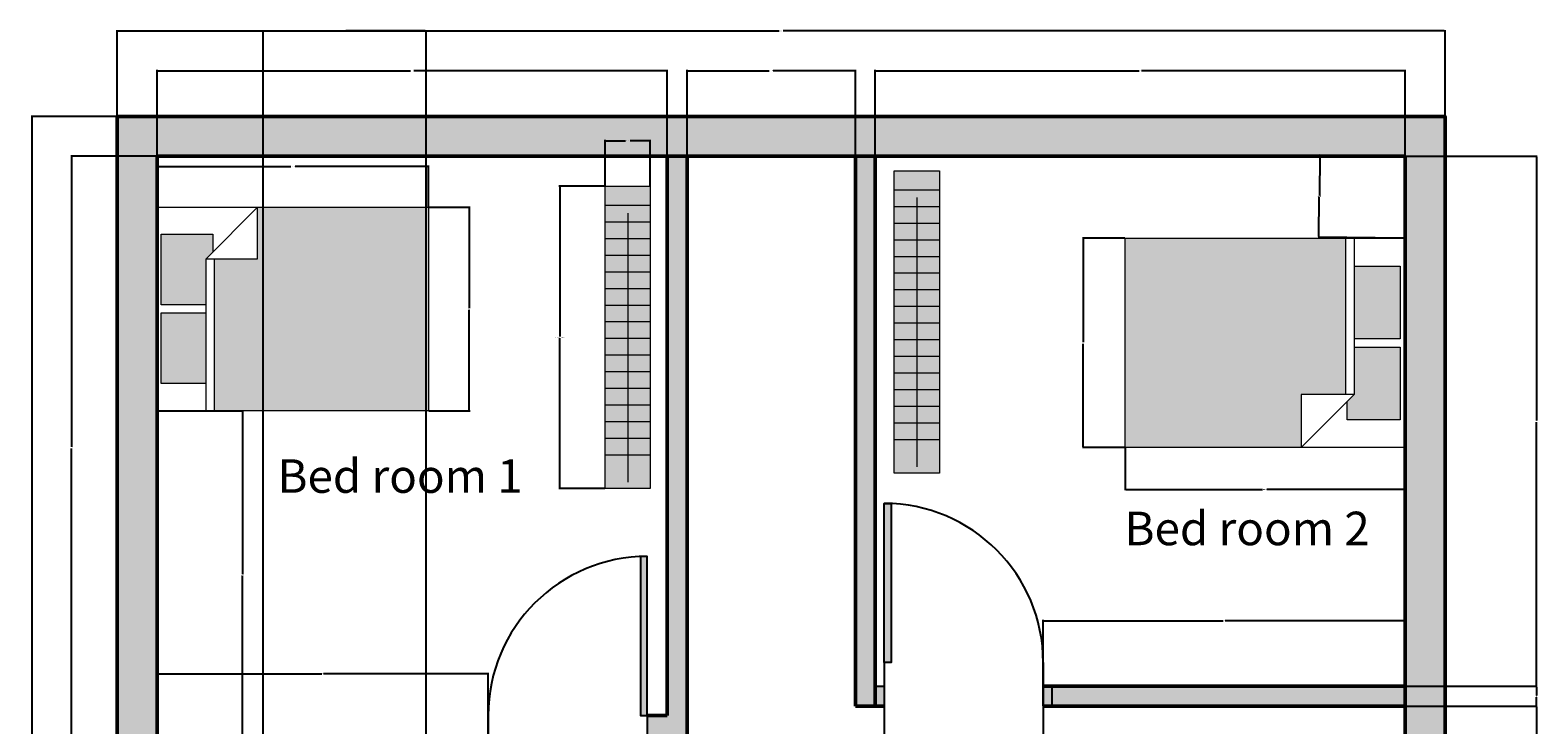
# Model space of a CAD drawing. Units: inches. Extents: x 2578 to 2919, y 51 to 451.
# Tile 5 of 5: x 2578 to 2919, y 293 to 451. Entities that reach past the tile are written whole.
import ezdxf

# ---------------------------------------------------------------- set-up
doc = ezdxf.new("R2010")
doc.units = ezdxf.units.IN
for name, color, linetype, lineweight in [('A-ANNO-DIMS', 2, 'Continuous', 18), ('A-AREA-IDEN', 7, 'Continuous', 25), ('A-DOOR', 4, 'Continuous', 25), ('A-FURN', 8, 'Continuous', 18), ('A-FURN-PATT', 253, 'Continuous', 13), ('A-WALL', 7, 'Continuous', 50), ('A-WALL-PATT', 250, 'Continuous', 13)]:
    doc.layers.add(name, color=color, linetype=linetype, lineweight=lineweight)
doc.layers.add('A-DOOR-PATT', color=29, linetype='Continuous', lineweight=13, true_color=0x4f342a)
doc.styles.get("Standard").update_dxf_attribs({"font": 'arial.ttf'})
doc.dimstyles.get("Standard").update_dxf_attribs({"dimtxt": 0.18, "dimasz": 0.18, "dimexe": 0.18, "dimexo": 0.0625, "dimgap": 0.09, "dimtad": 0, "dimtih": 1, "dimtoh": 1, "dimdec": 4, "dimzin": 0, "dimdsep": 46, "dimtxsty": 'Standard', "dimcen": 0.09, "dimadec": 0, "dimazin": 0, "dimtfac": 1, "dimtdec": 4, "dimtofl": 0, "dimtmove": 0, "dimatfit": 3, "dimfxl": 1, "dimtolj": 1, "dimtzin": 0, "dimarcsym": 0})

# ---------------------------------------------------------------- blocks, each defined once
blk = doc.blocks.new('*U3')
for p, q in [((0, 0), (0, -6)), ((40, 0), (40, -6))]:
    blk.add_line(p, q)
blk.add_lwpolyline([(0, 0), (0, 40), (1.75, 40), (1.75, 0)], close=True)
blk.add_arc((0, 0), 40, 0, 90)
blk = doc.blocks.new('*U2')
for p, q in [((0, 0), (0, -6)), ((-40, 0), (-40, -6))]:
    blk.add_line(p, q)
blk.add_lwpolyline([(0, 0), (0, 40), (-1.75, 40), (-1.75, 0)], close=True)
blk.add_arc((0, 0), 40, 90, 180)
blk = doc.blocks.new('Bed - Queen')
for p, q in [((0, -80.00003), (0, 0)), ((0, 0), (59.99999, 0)), ((59.99999, 0), (59.99999, -80.00003)), ((7.99999, -1.2), (28.79998, -1.2)), ((7.99999, -14.4), (7.99999, -1.2)), ((28.79998, -1.2), (28.79998, -14.4)), ((31.19999, -1.2), (51.99999, -1.2)), ((31.19999, -14.4), (31.19999, -1.2)), ((51.99999, -1.2), (51.99999, -16.4)), ((0, -14.4), (44.8, -14.4)), ((44.8, -16.8), (0, -16.8)), ((59.99999, -29.6), (44.8, -14.4)), ((44.8, -14.4), (44.8, -29.6)), ((51.99999, -16.4), (46.79936, -16.4)), ((44.8, -29.6), (59.99999, -29.6)), ((59.99999, -80.00003), (0, -80.00003))]:
    blk.add_line(p, q)
blk = doc.blocks.new('BEDROOM-SLATTED-UNIT')
for p, q in [((0, 0), (0, 68.46)), ((0, 68.46), (10.22, 68.46)), ((10.22, 68.46), (10.22, 0)), ((10.22, 64.08), (0, 64.08)), ((5.11, 62.36), (5.11, 1.41)), ((10.22, 60.31), (0, 60.31)), ((10.22, 56.54), (0, 56.54)), ((10.22, 52.77), (0, 52.77)), ((10.22, 49), (0, 49)), ((10.22, 45.23), (0, 45.23)), ((10.22, 41.46), (0, 41.46)), ((10.22, 37.7), (0, 37.7)), ((10.22, 33.93), (0, 33.93)), ((10.22, 30.16), (0, 30.16)), ((10.22, 26.39), (0, 26.39)), ((10.22, 22.62), (0, 22.62)), ((10.22, 18.85), (0, 18.85)), ((10.22, 15.08), (0, 15.08)), ((10.22, 11.31), (0, 11.31)), ((10.22, 7.54), (0, 7.54)), ((10.22, 0), (0, 0))]:
    blk.add_line(p, q)
blk = doc.blocks.new('*D15')
at = {"layer": 'A-ANNO-DIMS', "color": 0, "lineweight": -2, "transparency": 16777216}
for p, q in [((2606.58, 410.67), (2606.58, 420)), ((2668.03, 410.67), (2668.03, 420)), ((2606.76, 419.82), (2636.81, 419.82)), ((2667.85, 419.82), (2637.8, 419.82))]:
    blk.add_line(p, q, dxfattribs=at)
at = {"layer": 'A-ANNO-DIMS', "color": 0, "transparency": 16777216}
for points in [[(2606.76, 419.85), (2606.76, 419.79), (2606.58, 419.82)], [(2667.85, 419.85), (2667.85, 419.79), (2668.03, 419.82)]]:
    blk.add_solid(points, dxfattribs=at)
at = {"layer": 'Defpoints', "color": 0, "transparency": 16777216}
for p in [(2606.58, 419.82), (2606.58, 410.61), (2668.03, 410.61)]:
    blk.add_point(p, dxfattribs=at)
at = {"layer": 'A-ANNO-DIMS', "color": 0, "transparency": 16777216, "insert": (2637.31, 419.82), "char_height": 0.18, "attachment_point": 5}
blk.add_mtext('\\A1;BED 61', dxfattribs=at)
blk = doc.blocks.new('*D16')
at = {"layer": 'A-ANNO-DIMS', "color": 0, "lineweight": -2, "transparency": 16777216}
for p, q in [((2668.09, 410.61), (2677.43, 410.61)), ((2677.25, 410.43), (2677.25, 387.75)), ((2677.25, 364.7), (2677.25, 387.38)), ((2668.09, 364.52), (2677.43, 364.52))]:
    blk.add_line(p, q, dxfattribs=at)
at = {"layer": 'A-ANNO-DIMS', "color": 0, "transparency": 16777216}
for points in [[(2677.22, 410.43), (2677.28, 410.43), (2677.25, 410.61)], [(2677.22, 364.7), (2677.28, 364.7), (2677.25, 364.52)]]:
    blk.add_solid(points, dxfattribs=at)
at = {"layer": 'Defpoints', "color": 0, "transparency": 16777216}
for p in [(2668.03, 410.61), (2677.25, 410.61), (2668.03, 364.52)]:
    blk.add_point(p, dxfattribs=at)
at = {"layer": 'A-ANNO-DIMS', "color": 0, "transparency": 16777216, "insert": (2677.25, 387.57), "char_height": 0.18, "attachment_point": 5}
blk.add_mtext('\\A1;46', dxfattribs=at)
blk = doc.blocks.new('*D17')
at = {"layer": 'A-ANNO-DIMS', "color": 0, "lineweight": -2, "transparency": 16777216}
for p, q in [((2825.75, 356.09), (2825.75, 346.5)), ((2888.95, 356.09), (2888.95, 346.5)), ((2825.93, 346.68), (2856.84, 346.68)), ((2888.77, 346.68), (2857.86, 346.68))]:
    blk.add_line(p, q, dxfattribs=at)
at = {"layer": 'A-ANNO-DIMS', "color": 0, "transparency": 16777216}
for points in [[(2825.93, 346.71), (2825.93, 346.65), (2825.75, 346.68)], [(2888.77, 346.71), (2888.77, 346.65), (2888.95, 346.68)]]:
    blk.add_solid(points, dxfattribs=at)
at = {"layer": 'Defpoints', "color": 0, "transparency": 16777216}
for p in [(2825.75, 356.16), (2888.95, 356.16), (2888.95, 346.68)]:
    blk.add_point(p, dxfattribs=at)
at = {"layer": 'A-ANNO-DIMS', "color": 0, "transparency": 16777216, "insert": (2857.35, 346.68), "char_height": 0.18, "attachment_point": 5}
blk.add_mtext('\\A1;BED 63', dxfattribs=at)
blk = doc.blocks.new('*D18')
at = {"layer": 'A-ANNO-DIMS', "color": 0, "lineweight": -2, "transparency": 16777216}
for p, q in [((2825.69, 403.56), (2816.09, 403.56)), ((2816.27, 403.38), (2816.27, 380.04)), ((2816.27, 356.34), (2816.27, 379.68)), ((2825.69, 356.16), (2816.09, 356.16))]:
    blk.add_line(p, q, dxfattribs=at)
at = {"layer": 'A-ANNO-DIMS', "color": 0, "transparency": 16777216}
for points in [[(2816.24, 403.38), (2816.3, 403.38), (2816.27, 403.56)], [(2816.24, 356.34), (2816.3, 356.34), (2816.27, 356.16)]]:
    blk.add_solid(points, dxfattribs=at)
at = {"layer": 'Defpoints', "color": 0, "transparency": 16777216}
for p in [(2825.75, 403.56), (2816.27, 356.16), (2825.75, 356.16)]:
    blk.add_point(p, dxfattribs=at)
at = {"layer": 'A-ANNO-DIMS', "color": 0, "transparency": 16777216, "insert": (2816.27, 379.86), "char_height": 0.18, "attachment_point": 5}
blk.add_mtext('\\A1;47', dxfattribs=at)
blk = doc.blocks.new('*D19')
at = {"layer": 'A-ANNO-DIMS', "color": 0, "lineweight": -2, "transparency": 16777216}
for p, q in [((2707.95, 415.37), (2697.56, 415.37)), ((2697.74, 415.19), (2697.74, 381.32)), ((2697.74, 347.09), (2697.74, 380.95)), ((2707.95, 346.91), (2697.56, 346.91))]:
    blk.add_line(p, q, dxfattribs=at)
at = {"layer": 'A-ANNO-DIMS', "color": 0, "transparency": 16777216}
for points in [[(2697.71, 415.19), (2697.77, 415.19), (2697.74, 415.37)], [(2697.71, 347.09), (2697.77, 347.09), (2697.74, 346.91)]]:
    blk.add_solid(points, dxfattribs=at)
at = {"layer": 'Defpoints', "color": 0, "transparency": 16777216}
for p in [(2697.74, 415.37), (2708.01, 415.37), (2708.01, 346.91)]:
    blk.add_point(p, dxfattribs=at)
at = {"layer": 'A-ANNO-DIMS', "color": 0, "transparency": 16777216, "insert": (2697.74, 381.14), "char_height": 0.18, "attachment_point": 5}
blk.add_mtext('\\A1;SLATTED UNIT 68 TYP.', dxfattribs=at)
blk = doc.blocks.new('*D20')
at = {"layer": 'A-ANNO-DIMS', "color": 0, "lineweight": -2, "transparency": 16777216}
for p, q in [((2708.01, 415.43), (2708.01, 425.82)), ((2708.19, 425.64), (2712.6, 425.64)), ((2718.05, 425.64), (2713.64, 425.64)), ((2718.23, 415.43), (2718.23, 425.82))]:
    blk.add_line(p, q, dxfattribs=at)
at = {"layer": 'A-ANNO-DIMS', "color": 0, "transparency": 16777216}
for points in [[(2708.19, 425.67), (2708.19, 425.61), (2708.01, 425.64)], [(2718.05, 425.67), (2718.05, 425.61), (2718.23, 425.64)]]:
    blk.add_solid(points, dxfattribs=at)
at = {"layer": 'Defpoints', "color": 0, "transparency": 16777216}
for p in [(2718.23, 425.64), (2708.01, 415.37), (2718.23, 415.37)]:
    blk.add_point(p, dxfattribs=at)
at = {"layer": 'A-ANNO-DIMS', "color": 0, "transparency": 16777216, "insert": (2713.12, 425.64), "char_height": 0.18, "attachment_point": 5}
blk.add_mtext('\\A1;10 TYP.', dxfattribs=at)
blk = doc.blocks.new('*D35')
at = {"layer": 'A-ANNO-DIMS', "color": 0, "lineweight": -2, "transparency": 16777216}
for p, q in [((2597.55, 431.2), (2597.55, 450.67)), ((2898.18, 431.2), (2898.18, 450.67)), ((2597.73, 450.49), (2747.4, 450.49)), ((2898, 450.49), (2748.33, 450.49))]:
    blk.add_line(p, q, dxfattribs=at)
at = {"layer": 'A-ANNO-DIMS', "color": 0, "transparency": 16777216}
for points in [[(2597.73, 450.52), (2597.73, 450.46), (2597.55, 450.49)], [(2898, 450.52), (2898, 450.46), (2898.18, 450.49)]]:
    blk.add_solid(points, dxfattribs=at)
at = {"layer": 'Defpoints', "color": 0, "transparency": 16777216}
for p in [(2898.18, 450.49), (2597.55, 431.14), (2898.18, 431.14)]:
    blk.add_point(p, dxfattribs=at)
at = {"layer": 'A-ANNO-DIMS', "color": 0, "transparency": 16777216, "insert": (2747.86, 450.49), "char_height": 0.18, "attachment_point": 5}
blk.add_mtext('\\A1;300.63', dxfattribs=at)
blk = doc.blocks.new('*D36')
at = {"layer": 'A-ANNO-DIMS', "color": 0, "lineweight": -2, "transparency": 16777216}
for p, q in [((2597.48, 431.14), (2578.02, 431.14)), ((2578.2, 430.96), (2578.2, 252.3)), ((2578.2, 73.28), (2578.2, 251.94)), ((2597.48, 73.1), (2578.02, 73.1))]:
    blk.add_line(p, q, dxfattribs=at)
at = {"layer": 'A-ANNO-DIMS', "color": 0, "transparency": 16777216}
for points in [[(2578.17, 430.96), (2578.23, 430.96), (2578.2, 431.14)], [(2578.17, 73.28), (2578.23, 73.28), (2578.2, 73.1)]]:
    blk.add_solid(points, dxfattribs=at)
at = {"layer": 'Defpoints', "color": 0, "transparency": 16777216}
for p in [(2578.2, 431.14), (2597.55, 431.14), (2597.55, 73.1)]:
    blk.add_point(p, dxfattribs=at)
at = {"layer": 'A-ANNO-DIMS', "color": 0, "transparency": 16777216, "insert": (2578.2, 252.12), "char_height": 0.18, "attachment_point": 5}
blk.add_mtext('\\A1;358.04', dxfattribs=at)
blk = doc.blocks.new('*D37')
at = {"layer": 'A-ANNO-DIMS', "color": 0, "lineweight": -2, "transparency": 16777216}
for p, q in [((2606.55, 422.2), (2606.55, 441.67)), ((2606.73, 441.49), (2663.91, 441.49)), ((2721.87, 441.49), (2664.68, 441.49)), ((2722.05, 422.2), (2722.05, 441.67))]:
    blk.add_line(p, q, dxfattribs=at)
at = {"layer": 'A-ANNO-DIMS', "color": 0, "transparency": 16777216}
for points in [[(2606.73, 441.52), (2606.73, 441.46), (2606.55, 441.49)], [(2721.87, 441.52), (2721.87, 441.46), (2722.05, 441.49)]]:
    blk.add_solid(points, dxfattribs=at)
at = {"layer": 'Defpoints', "color": 0, "transparency": 16777216}
for p in [(2722.05, 441.49), (2606.55, 422.14), (2722.05, 422.14)]:
    blk.add_point(p, dxfattribs=at)
at = {"layer": 'A-ANNO-DIMS', "color": 0, "transparency": 16777216, "insert": (2664.3, 441.49), "char_height": 0.18, "attachment_point": 5}
blk.add_mtext('\\A1;115.5', dxfattribs=at)
blk = doc.blocks.new('*D38')
at = {"layer": 'A-ANNO-DIMS', "color": 0, "lineweight": -2, "transparency": 16777216}
for p, q in [((2726.55, 422.2), (2726.55, 441.67)), ((2726.73, 441.49), (2745.15, 441.49)), ((2764.5, 441.49), (2746.08, 441.49)), ((2764.68, 422.2), (2764.68, 441.67))]:
    blk.add_line(p, q, dxfattribs=at)
at = {"layer": 'A-ANNO-DIMS', "color": 0, "transparency": 16777216}
for points in [[(2726.73, 441.52), (2726.73, 441.46), (2726.55, 441.49)], [(2764.5, 441.52), (2764.5, 441.46), (2764.68, 441.49)]]:
    blk.add_solid(points, dxfattribs=at)
at = {"layer": 'Defpoints', "color": 0, "transparency": 16777216}
for p in [(2764.68, 441.49), (2726.55, 422.14), (2764.68, 422.14)]:
    blk.add_point(p, dxfattribs=at)
at = {"layer": 'A-ANNO-DIMS', "color": 0, "transparency": 16777216, "insert": (2745.61, 441.49), "char_height": 0.18, "attachment_point": 5}
blk.add_mtext('\\A1;38.134', dxfattribs=at)
blk = doc.blocks.new('*D39')
at = {"layer": 'A-ANNO-DIMS', "color": 0, "lineweight": -2, "transparency": 16777216}
for p, q in [((2769.18, 422.2), (2769.18, 441.67)), ((2769.36, 441.49), (2828.9, 441.49)), ((2889, 441.49), (2829.46, 441.49)), ((2889.18, 422.2), (2889.18, 441.67))]:
    blk.add_line(p, q, dxfattribs=at)
at = {"layer": 'A-ANNO-DIMS', "color": 0, "transparency": 16777216}
for points in [[(2769.36, 441.52), (2769.36, 441.46), (2769.18, 441.49)], [(2889, 441.52), (2889, 441.46), (2889.18, 441.49)]]:
    blk.add_solid(points, dxfattribs=at)
at = {"layer": 'Defpoints', "color": 0, "transparency": 16777216}
for p in [(2889.18, 441.49), (2769.18, 422.14), (2889.18, 422.14)]:
    blk.add_point(p, dxfattribs=at)
at = {"layer": 'A-ANNO-DIMS', "color": 0, "transparency": 16777216, "insert": (2829.18, 441.49), "char_height": 0.18, "attachment_point": 5}
blk.add_mtext('\\A1;120', dxfattribs=at)
blk = doc.blocks.new('*D40')
at = {"layer": 'A-ANNO-DIMS', "color": 0, "lineweight": -2, "transparency": 16777216}
for p, q in [((2606.48, 422.14), (2587.02, 422.14)), ((2587.2, 421.96), (2587.2, 356.32)), ((2587.2, 290.32), (2587.2, 355.96)), ((2606.48, 290.14), (2587.02, 290.14))]:
    blk.add_line(p, q, dxfattribs=at)
at = {"layer": 'A-ANNO-DIMS', "color": 0, "transparency": 16777216}
for points in [[(2587.17, 421.96), (2587.23, 421.96), (2587.2, 422.14)], [(2587.17, 290.32), (2587.23, 290.32), (2587.2, 290.14)]]:
    blk.add_solid(points, dxfattribs=at)
at = {"layer": 'Defpoints', "color": 0, "transparency": 16777216}
for p in [(2587.2, 422.14), (2606.55, 422.14), (2606.55, 290.14)]:
    blk.add_point(p, dxfattribs=at)
at = {"layer": 'A-ANNO-DIMS', "color": 0, "transparency": 16777216, "insert": (2587.2, 356.14), "char_height": 0.18, "attachment_point": 5}
blk.add_mtext('\\A1;132', dxfattribs=at)
blk = doc.blocks.new('*D41')
at = {"layer": 'A-ANNO-DIMS', "color": 0, "lineweight": -2, "transparency": 16777216}
for p, q in [((2889.24, 422.14), (2919.06, 422.14)), ((2918.88, 421.96), (2918.88, 362.32)), ((2918.88, 302.32), (2918.88, 361.96)), ((2889.24, 302.14), (2919.06, 302.14))]:
    blk.add_line(p, q, dxfattribs=at)
at = {"layer": 'A-ANNO-DIMS', "color": 0, "transparency": 16777216}
for points in [[(2918.85, 421.96), (2918.91, 421.96), (2918.88, 422.14)], [(2918.85, 302.32), (2918.91, 302.32), (2918.88, 302.14)]]:
    blk.add_solid(points, dxfattribs=at)
at = {"layer": 'Defpoints', "color": 0, "transparency": 16777216}
for p in [(2889.18, 422.14), (2918.88, 422.14), (2889.18, 302.14)]:
    blk.add_point(p, dxfattribs=at)
at = {"layer": 'A-ANNO-DIMS', "color": 0, "transparency": 16777216, "insert": (2918.88, 362.14), "char_height": 0.18, "attachment_point": 5}
blk.add_mtext('\\A1;120', dxfattribs=at)
blk = doc.blocks.new('*D49')
at = {"layer": 'A-ANNO-DIMS', "color": 0, "lineweight": -2, "transparency": 16777216}
for p, q in [((2889.24, 297.64), (2919.06, 297.64)), ((2918.88, 297.46), (2918.88, 254.31)), ((2918.88, 210.79), (2918.88, 253.94)), ((2889.24, 210.61), (2919.06, 210.61))]:
    blk.add_line(p, q, dxfattribs=at)
at = {"layer": 'A-ANNO-DIMS', "color": 0, "transparency": 16777216}
for points in [[(2918.85, 297.46), (2918.91, 297.46), (2918.88, 297.64)], [(2918.85, 210.79), (2918.91, 210.79), (2918.88, 210.61)]]:
    blk.add_solid(points, dxfattribs=at)
at = {"layer": 'Defpoints', "color": 0, "transparency": 16777216}
for p in [(2889.18, 297.64), (2918.88, 297.64), (2889.18, 210.61)]:
    blk.add_point(p, dxfattribs=at)
at = {"layer": 'A-ANNO-DIMS', "color": 0, "transparency": 16777216, "insert": (2918.88, 254.13), "char_height": 0.18, "attachment_point": 5}
blk.add_mtext('\\A1;87.03', dxfattribs=at)
blk = doc.blocks.new('*D53')
at = {"layer": 'A-ANNO-DIMS', "color": 0, "lineweight": -2, "transparency": 16777216}
for p, q in [((2606.55, 285.7), (2606.55, 305.17)), ((2606.73, 304.99), (2643.83, 304.99)), ((2681.37, 304.99), (2644.27, 304.99)), ((2681.55, 285.7), (2681.55, 305.17))]:
    blk.add_line(p, q, dxfattribs=at)
at = {"layer": 'A-ANNO-DIMS', "color": 0, "transparency": 16777216}
for points in [[(2606.73, 305.02), (2606.73, 304.96), (2606.55, 304.99)], [(2681.37, 305.02), (2681.37, 304.96), (2681.55, 304.99)]]:
    blk.add_solid(points, dxfattribs=at)
at = {"layer": 'Defpoints', "color": 0, "transparency": 16777216}
for p in [(2681.55, 304.99), (2606.55, 285.64), (2681.55, 285.64)]:
    blk.add_point(p, dxfattribs=at)
at = {"layer": 'A-ANNO-DIMS', "color": 0, "transparency": 16777216, "insert": (2644.05, 304.99), "char_height": 0.18, "attachment_point": 5}
blk.add_mtext('\\A1;75', dxfattribs=at)
blk = doc.blocks.new('*D54')
at = {"layer": 'A-ANNO-DIMS', "color": 0, "lineweight": -2, "transparency": 16777216}
for p, q in [((2771.18, 297.58), (2771.18, 278.11)), ((2807.18, 297.58), (2807.18, 278.11)), ((2771.36, 278.29), (2788.96, 278.29)), ((2807, 278.29), (2789.4, 278.29))]:
    blk.add_line(p, q, dxfattribs=at)
at = {"layer": 'A-ANNO-DIMS', "color": 0, "transparency": 16777216}
for points in [[(2771.36, 278.32), (2771.36, 278.26), (2771.18, 278.29)], [(2807, 278.32), (2807, 278.26), (2807.18, 278.29)]]:
    blk.add_solid(points, dxfattribs=at)
at = {"layer": 'Defpoints', "color": 0, "transparency": 16777216}
for p in [(2771.18, 297.64), (2807.18, 297.64), (2771.18, 278.29)]:
    blk.add_point(p, dxfattribs=at)
at = {"layer": 'A-ANNO-DIMS', "color": 0, "transparency": 16777216, "insert": (2789.18, 278.29), "char_height": 0.18, "attachment_point": 5}
blk.add_mtext('\\A1;36', dxfattribs=at)
blk = doc.blocks.new('*D55')
at = {"layer": 'A-ANNO-DIMS', "color": 0, "lineweight": -2, "transparency": 16777216}
for p, q in [((2807.18, 297.7), (2807.18, 317.17)), ((2807.36, 316.99), (2847.96, 316.99)), ((2889, 316.99), (2848.4, 316.99)), ((2889.18, 297.7), (2889.18, 317.17))]:
    blk.add_line(p, q, dxfattribs=at)
at = {"layer": 'A-ANNO-DIMS', "color": 0, "transparency": 16777216}
for points in [[(2807.36, 317.02), (2807.36, 316.96), (2807.18, 316.99)], [(2889, 317.02), (2889, 316.96), (2889.18, 316.99)]]:
    blk.add_solid(points, dxfattribs=at)
at = {"layer": 'Defpoints', "color": 0, "transparency": 16777216}
for p in [(2889.18, 316.99), (2807.18, 297.64), (2889.18, 297.64)]:
    blk.add_point(p, dxfattribs=at)
at = {"layer": 'A-ANNO-DIMS', "color": 0, "transparency": 16777216, "insert": (2848.18, 316.99), "char_height": 0.18, "attachment_point": 5}
blk.add_mtext('\\A1;82', dxfattribs=at)
blk = doc.blocks.new('*D61')
at = {"layer": 'A-ANNO-DIMS', "color": 0, "lineweight": -2, "transparency": 16777216}
for p, q in [((2889.24, 302.14), (2919.06, 302.14)), ((2918.88, 301.96), (2918.88, 300.07)), ((2889.24, 297.64), (2919.06, 297.64)), ((2918.88, 297.82), (2918.88, 299.71))]:
    blk.add_line(p, q, dxfattribs=at)
at = {"layer": 'A-ANNO-DIMS', "color": 0, "transparency": 16777216}
for points in [[(2918.85, 301.96), (2918.91, 301.96), (2918.88, 302.14)], [(2918.85, 297.82), (2918.91, 297.82), (2918.88, 297.64)]]:
    blk.add_solid(points, dxfattribs=at)
at = {"layer": 'Defpoints', "color": 0, "transparency": 16777216}
for p in [(2889.18, 302.14), (2918.88, 302.14), (2889.18, 297.64)]:
    blk.add_point(p, dxfattribs=at)
at = {"layer": 'A-ANNO-DIMS', "color": 0, "transparency": 16777216, "insert": (2918.88, 299.89), "char_height": 0.18, "attachment_point": 5}
blk.add_mtext('\\A1;4.5', dxfattribs=at)
blk = doc.blocks.new('*D70')
at = {"layer": 'A-ANNO-DIMS', "color": 0, "lineweight": -2, "transparency": 16777216}
for p, q in [((2630.55, 156.2), (2630.55, 450.67)), ((2667.45, 155.71), (2667.45, 450.67)), ((2630.73, 450.49), (2648.67, 450.49)), ((2667.27, 450.49), (2649.32, 450.49))]:
    blk.add_line(p, q, dxfattribs=at)
at = {"layer": 'A-ANNO-DIMS', "color": 0, "transparency": 16777216}
for points in [[(2630.73, 450.52), (2630.73, 450.46), (2630.55, 450.49)], [(2667.27, 450.52), (2667.27, 450.46), (2667.45, 450.49)]]:
    blk.add_solid(points, dxfattribs=at)
at = {"layer": 'Defpoints', "color": 0, "transparency": 16777216}
for p in [(2667.45, 450.49), (2630.55, 156.14), (2667.45, 155.64)]:
    blk.add_point(p, dxfattribs=at)
at = {"layer": 'A-ANNO-DIMS', "color": 0, "transparency": 16777216, "insert": (2649, 450.49), "char_height": 0.18, "attachment_point": 5}
blk.add_mtext('\\A1;36.9', dxfattribs=at)
blk = doc.blocks.new('*D72')
at = {"layer": 'A-ANNO-DIMS', "color": 0, "lineweight": -2, "transparency": 16777216}
for p, q in [((2606.65, 364.52), (2626.11, 364.51)), ((2625.93, 364.33), (2625.91, 327.5)), ((2625.9, 290.31), (2625.91, 327.14)), ((2606.61, 290.14), (2626.08, 290.13))]:
    blk.add_line(p, q, dxfattribs=at)
at = {"layer": 'A-ANNO-DIMS', "color": 0, "transparency": 16777216}
for points in [[(2625.9, 364.33), (2625.96, 364.33), (2625.93, 364.51)], [(2625.87, 290.31), (2625.93, 290.31), (2625.9, 290.13)]]:
    blk.add_solid(points, dxfattribs=at)
at = {"layer": 'Defpoints', "color": 0, "transparency": 16777216}
for p in [(2606.58, 364.52), (2606.55, 290.14), (2625.9, 290.13)]:
    blk.add_point(p, dxfattribs=at)
at = {"layer": 'A-ANNO-DIMS', "color": 0, "transparency": 16777216, "insert": (2625.91, 327.32), "char_height": 0.18, "attachment_point": 5}
blk.add_mtext('\\A1;74.38', dxfattribs=at)
blk = doc.blocks.new('*D73')
at = {"layer": 'A-ANNO-DIMS', "color": 0, "lineweight": -2, "transparency": 16777216}
for p, q in [((2889.12, 422.14), (2869.65, 422.39)), ((2869.83, 422.2), (2869.72, 413.27)), ((2869.6, 403.98), (2869.71, 412.91)), ((2888.88, 403.56), (2869.42, 403.8))]:
    blk.add_line(p, q, dxfattribs=at)
at = {"layer": 'A-ANNO-DIMS', "color": 0, "transparency": 16777216}
for points in [[(2869.8, 422.2), (2869.86, 422.2), (2869.83, 422.38)], [(2869.57, 403.98), (2869.63, 403.98), (2869.6, 403.8)]]:
    blk.add_solid(points, dxfattribs=at)
at = {"layer": 'Defpoints', "color": 0, "transparency": 16777216}
for p in [(2869.83, 422.38), (2889.18, 422.14), (2888.95, 403.56)]:
    blk.add_point(p, dxfattribs=at)
at = {"layer": 'A-ANNO-DIMS', "color": 0, "transparency": 16777216, "insert": (2869.72, 413.09), "char_height": 0.18, "attachment_point": 5}
blk.add_mtext('\\A1;18.586', dxfattribs=at)

msp = doc.modelspace()

# ---------------------------------------------------------------- hatches: boundary and pattern name
at = {"layer": 'A-DOOR-PATT'}
h = msp.add_hatch(color=256, dxfattribs=at)
h.dxf.hatch_style = 1
h.paths.add_polyline_path([(2717.5545, 331.5492, 0.01094143), (2715.9791, 331.5147), (2715.9791, 295.5417), (2717.5545, 295.5417)])
h.paths.add_polyline_path([(2772.7563, 343.5147, 0.01094143), (2771.181, 343.5492), (2771.181, 307.5417), (2772.7563, 307.5417)])
h.paths.add_polyline_path([(2809.181, 302.1406), (2807.181, 302.1406), (2807.181, 297.6406), (2809.181, 297.6406)])
h.paths.add_polyline_path([(2681.547, 290.1406), (2679.547, 290.1406), (2679.547, 285.6406), (2681.547, 285.6406)])
h.paths.add_polyline_path([(2870.5896, 193.5988), (2834.5821, 193.5988), (2834.5821, 192.0235), (2870.5551, 192.0235, 0.01094143)])
h.paths.add_polyline_path([(2829.181, 157.5988), (2824.681, 157.5988), (2824.681, 155.5988), (2829.181, 155.5988)])
h.paths.add_polyline_path([(2702.547, 145.6406), (2698.047, 145.6406), (2698.047, 143.6481), (2702.547, 143.6481)])
h.paths.add_polyline_path([(2697.1459, 109.2159), (2661.1384, 109.2159), (2661.1384, 107.6406), (2697.1459, 107.6406)])
h.paths.add_polyline_path([(2702.547, 107.6406), (2698.047, 107.6406), (2698.047, 105.6406), (2702.547, 105.6406)])
h.paths.add_polyline_path([(2771.181, 302.1406), (2769.181, 302.1406), (2769.181, 297.6406), (2771.181, 297.6406)])
at = {"layer": 'A-FURN-PATT'}
h = msp.add_hatch(color=256, dxfattribs=at)
h.dxf.hatch_style = 1
h.paths.add_polyline_path([(2708.0083, 354.4474), (2708.0083, 346.9083), (2718.2265, 346.9083), (2718.2265, 354.4474)])
h.paths.add_polyline_path([(2718.2265, 358.2169), (2713.1174, 358.2169), (2713.1174, 354.4474), (2718.2265, 354.4474)])
h.paths.add_polyline_path([(2713.1174, 358.2169), (2708.0083, 358.2169), (2708.0083, 354.4474), (2713.1174, 354.4474)])
h.paths.add_polyline_path([(2713.1174, 361.9865), (2708.0083, 361.9865), (2708.0083, 358.2169), (2713.1174, 358.2169)])
h.paths.add_polyline_path([(2718.2265, 361.9865), (2713.1174, 361.9865), (2713.1174, 358.2169), (2718.2265, 358.2169)])
h.paths.add_polyline_path([(2718.2265, 365.756), (2713.1174, 365.756), (2713.1174, 361.9865), (2718.2265, 361.9865)])
h.paths.add_polyline_path([(2713.1174, 365.756), (2708.0083, 365.756), (2708.0083, 361.9865), (2713.1174, 361.9865)])
h.paths.add_polyline_path([(2713.1174, 369.5255), (2708.0083, 369.5255), (2708.0083, 365.756), (2713.1174, 365.756)])
h.paths.add_polyline_path([(2718.2265, 369.5255), (2713.1174, 369.5255), (2713.1174, 365.756), (2718.2265, 365.756)])
h.paths.add_polyline_path([(2718.2265, 373.2951), (2713.1174, 373.2951), (2713.1174, 369.5255), (2718.2265, 369.5255)])
h.paths.add_polyline_path([(2713.1174, 373.2951), (2708.0083, 373.2951), (2708.0083, 369.5255), (2713.1174, 369.5255)])
h.paths.add_polyline_path([(2713.1174, 377.0646), (2708.0083, 377.0646), (2708.0083, 373.2951), (2713.1174, 373.2951)])
h.paths.add_polyline_path([(2718.2265, 377.0646), (2713.1174, 377.0646), (2713.1174, 373.2951), (2718.2265, 373.2951)])
h.paths.add_polyline_path([(2718.2265, 380.8341), (2713.1174, 380.8341), (2713.1174, 377.0646), (2718.2265, 377.0646)])
h.paths.add_polyline_path([(2713.1174, 380.8341), (2708.0083, 380.8341), (2708.0083, 377.0646), (2713.1174, 377.0646)])
h.paths.add_polyline_path([(2713.1174, 384.6037), (2708.0083, 384.6037), (2708.0083, 380.8341), (2713.1174, 380.8341)])
h.paths.add_polyline_path([(2718.2265, 384.6037), (2713.1174, 384.6037), (2713.1174, 380.8341), (2718.2265, 380.8341)])
h.paths.add_polyline_path([(2718.2265, 388.3732), (2713.1174, 388.3732), (2713.1174, 384.6037), (2718.2265, 384.6037)])
h.paths.add_polyline_path([(2713.1174, 388.3732), (2708.0083, 388.3732), (2708.0083, 384.6037), (2713.1174, 384.6037)])
h.paths.add_polyline_path([(2713.1174, 392.1427), (2708.0083, 392.1427), (2708.0083, 388.3732), (2713.1174, 388.3732)])
h.paths.add_polyline_path([(2718.2265, 392.1427), (2713.1174, 392.1427), (2713.1174, 388.3732), (2718.2265, 388.3732)])
h.paths.add_polyline_path([(2718.2265, 395.9123), (2713.1174, 395.9123), (2713.1174, 392.1427), (2718.2265, 392.1427)])
h.paths.add_polyline_path([(2713.1174, 395.9123), (2708.0083, 395.9123), (2708.0083, 392.1427), (2713.1174, 392.1427)])
h.paths.add_polyline_path([(2713.1174, 399.6818), (2708.0083, 399.6818), (2708.0083, 395.9123), (2713.1174, 395.9123)])
h.paths.add_polyline_path([(2718.2265, 399.6818), (2713.1174, 399.6818), (2713.1174, 395.9123), (2718.2265, 395.9123)])
h.paths.add_polyline_path([(2718.2265, 403.4513), (2713.1174, 403.4513), (2713.1174, 399.6818), (2718.2265, 399.6818)])
h.paths.add_polyline_path([(2713.1174, 403.4513), (2708.0083, 403.4513), (2708.0083, 399.6818), (2713.1174, 399.6818)])
h.paths.add_polyline_path([(2713.1174, 407.2209), (2708.0083, 407.2209), (2708.0083, 403.4513), (2713.1174, 403.4513)])
h.paths.add_polyline_path([(2718.2265, 407.2209), (2713.1174, 407.2209), (2713.1174, 403.4513), (2718.2265, 403.4513)])
h.paths.add_polyline_path([(2718.2265, 410.9904), (2708.0083, 410.9904), (2708.0083, 407.2209), (2718.2265, 407.2209)])
h.paths.add_polyline_path([(2718.2265, 415.3677), (2708.0083, 415.3677), (2708.0083, 410.9904), (2718.2265, 410.9904)])
h.paths.add_polyline_path([(2773.4812, 357.9317), (2773.4812, 350.3927), (2783.6994, 350.3927), (2783.6994, 357.9317)])
h.paths.add_polyline_path([(2778.5903, 361.7013), (2773.4812, 361.7013), (2773.4812, 357.9317), (2778.5903, 357.9317)])
h.paths.add_polyline_path([(2778.5903, 365.4708), (2773.4812, 365.4708), (2773.4812, 361.7013), (2778.5903, 361.7013)])
h.paths.add_polyline_path([(2778.5903, 373.0099), (2773.4812, 373.0099), (2773.4812, 369.2404), (2778.5903, 369.2404)])
h.paths.add_polyline_path([(2778.5903, 369.2404), (2773.4812, 369.2404), (2773.4812, 365.4708), (2778.5903, 365.4708)])
h.paths.add_polyline_path([(2783.6994, 369.2404), (2778.5903, 369.2404), (2778.5903, 365.4708), (2783.6994, 365.4708)])
h.paths.add_polyline_path([(2783.6994, 365.4708), (2778.5903, 365.4708), (2778.5903, 361.7013), (2783.6994, 361.7013)])
h.paths.add_polyline_path([(2783.6994, 361.7013), (2778.5903, 361.7013), (2778.5903, 357.9317), (2783.6994, 357.9317)])
h.paths.add_polyline_path([(2783.6994, 373.0099), (2778.5903, 373.0099), (2778.5903, 369.2404), (2783.6994, 369.2404)])
h.paths.add_polyline_path([(2783.6994, 376.7794), (2778.5903, 376.7794), (2778.5903, 373.0099), (2783.6994, 373.0099)])
h.paths.add_polyline_path([(2778.5903, 376.7794), (2773.4812, 376.7794), (2773.4812, 373.0099), (2778.5903, 373.0099)])
h.paths.add_polyline_path([(2778.5903, 380.549), (2773.4812, 380.549), (2773.4812, 376.7794), (2778.5903, 376.7794)])
h.paths.add_polyline_path([(2783.6994, 380.549), (2778.5903, 380.549), (2778.5903, 376.7794), (2783.6994, 376.7794)])
h.paths.add_polyline_path([(2783.6994, 384.3185), (2778.5903, 384.3185), (2778.5903, 380.549), (2783.6994, 380.549)])
h.paths.add_polyline_path([(2778.5903, 384.3185), (2773.4812, 384.3185), (2773.4812, 380.549), (2778.5903, 380.549)])
h.paths.add_polyline_path([(2778.5903, 388.088), (2773.4812, 388.088), (2773.4812, 384.3185), (2778.5903, 384.3185)])
h.paths.add_polyline_path([(2783.6994, 388.088), (2778.5903, 388.088), (2778.5903, 384.3185), (2783.6994, 384.3185)])
h.paths.add_polyline_path([(2783.6994, 391.8576), (2778.5903, 391.8576), (2778.5903, 388.088), (2783.6994, 388.088)])
h.paths.add_polyline_path([(2778.5903, 391.8576), (2773.4812, 391.8576), (2773.4812, 388.088), (2778.5903, 388.088)])
h.paths.add_polyline_path([(2778.5903, 395.6271), (2773.4812, 395.6271), (2773.4812, 391.8576), (2778.5903, 391.8576)])
h.paths.add_polyline_path([(2783.6994, 395.6271), (2778.5903, 395.6271), (2778.5903, 391.8576), (2783.6994, 391.8576)])
h.paths.add_polyline_path([(2783.6994, 399.3966), (2778.5903, 399.3966), (2778.5903, 395.6271), (2783.6994, 395.6271)])
h.paths.add_polyline_path([(2778.5903, 399.3966), (2773.4812, 399.3966), (2773.4812, 395.6271), (2778.5903, 395.6271)])
h.paths.add_polyline_path([(2778.5903, 403.1662), (2773.4812, 403.1662), (2773.4812, 399.3966), (2778.5903, 399.3966)])
h.paths.add_polyline_path([(2783.6994, 403.1662), (2778.5903, 403.1662), (2778.5903, 399.3966), (2783.6994, 399.3966)])
h.paths.add_polyline_path([(2783.6994, 406.9357), (2778.5903, 406.9357), (2778.5903, 403.1662), (2783.6994, 403.1662)])
h.paths.add_polyline_path([(2778.5903, 406.9357), (2773.4812, 406.9357), (2773.4812, 403.1662), (2778.5903, 403.1662)])
h.paths.add_polyline_path([(2778.5903, 410.7052), (2773.4812, 410.7052), (2773.4812, 406.9357), (2778.5903, 406.9357)])
h.paths.add_polyline_path([(2783.6994, 410.7052), (2778.5903, 410.7052), (2778.5903, 406.9357), (2783.6994, 406.9357)])
h.paths.add_polyline_path([(2783.6994, 414.4748), (2773.4812, 414.4748), (2773.4812, 410.7052), (2783.6994, 410.7052)])
h.paths.add_polyline_path([(2783.6994, 418.8521), (2773.4812, 418.8521), (2773.4812, 414.4748), (2783.6994, 414.4748)])
h = msp.add_hatch(color=256, dxfattribs=at)
h.dxf.hatch_style = 1
h.paths.add_polyline_path([(2668.0284, 410.6078), (2629.3175, 410.6078), (2629.3175, 398.9331), (2619.4862, 398.9331), (2619.4862, 364.5234), (2668.0284, 364.5234)])
h.paths.add_polyline_path([(2617.6428, 398.9331), (2619.1789, 400.4692), (2619.1789, 404.4632), (2607.5042, 404.4632), (2607.5042, 388.4873), (2617.6428, 388.4873)])
h.paths.add_polyline_path([(2617.6428, 386.6439), (2607.5042, 386.6439), (2607.5042, 370.668), (2617.6428, 370.668)])
h.paths.add_polyline_path([(2875.6753, 403.5558), (2825.7487, 403.5558), (2825.7487, 356.1571), (2865.5636, 356.1571), (2865.5636, 368.1648), (2875.6753, 368.1648)])
h.paths.add_polyline_path([(2887.999, 397.2359), (2877.5713, 397.2359), (2877.5713, 380.8044), (2887.999, 380.8044)])
h.paths.add_polyline_path([(2887.999, 378.9085), (2877.5713, 378.9085), (2877.5713, 368.1648), (2875.9913, 366.5848), (2875.9913, 362.4769), (2887.999, 362.4769)])
h.paths.add_polyline_path([(2863.3609, 291.2749), (2850.0358, 291.2749), (2849.9056, 290.442), (2863.4911, 290.442)])
h.paths.add_polyline_path([(2834.6285, 271.8336), (2833.7957, 271.7035), (2833.7957, 258.3783), (2834.6285, 258.2482)])
h.paths.add_polyline_path([(2834.6285, 248.5146), (2833.7957, 248.3844), (2833.7957, 235.0593), (2834.6285, 234.9291)])
h.paths.add_polyline_path([(2879.601, 248.3844), (2878.7682, 248.5146), (2878.7682, 234.9291), (2879.601, 235.0593)])
h.paths.add_polyline_path([(2879.601, 271.7035), (2878.7682, 271.8336), (2878.7682, 258.2482), (2879.601, 258.3783)])
h.paths.add_polyline_path([(2863.4911, 216.3207), (2849.9056, 216.3207), (2850.0358, 215.4879), (2863.3609, 215.4879)])
h.paths.add_polyline_path([(2875.3365, 114.2473, 0.48007965), (2857.7894, 112.0785, 0.21500378), (2857.7543, 108.7906, 0.4800795), (2875.2511, 106.2478)])
h.paths.add_polyline_path([(2880.9002, 120.1884), (2879.9002, 120.199), (2879.8682, 117.1992), (2881.3682, 117.1832), (2881.3788, 118.1831), (2880.8789, 118.1885)])
h.paths.add_polyline_path([(2888.3838, 118.6084, 0.50000012), (2887.3945, 119.619), (2883.3947, 119.6617, 0.50000012), (2882.3841, 118.6724), (2882.2027, 101.6734, 0.50000012), (2883.192, 100.6628), (2887.1918, 100.6201, 0.50000012), (2888.2024, 101.6094)])
at = {"layer": 'A-WALL-PATT'}
h = msp.add_hatch(color=256, dxfattribs=at)
h.dxf.hatch_style = 1
h.paths.add_polyline_path([(2606.547, 422.1406), (2889.181, 422.1406), (2889.181, 210.611), (2824.681, 210.611), (2824.681, 193.5988), (2829.181, 193.5988), (2829.181, 206.111), (2889.181, 206.111), (2889.181, 99.5988), (2829.181, 99.5988), (2829.181, 155.5988), (2824.681, 155.5988), (2824.681, 95.0988), (2889.181, 95.0988), (2889.181, 82.1022), (2762.547, 82.1022), (2762.547, 73.1022), (2898.181, 73.1022), (2898.181, 233.1022), (2898.181, 431.1406), (2597.547, 431.1406), (2597.547, 73.1022), (2726.547, 73.1022), (2726.547, 82.1022), (2606.547, 82.1022), (2606.547, 173.1406), (2698.047, 173.1406), (2698.047, 145.6406), (2702.547, 145.6406), (2702.547, 157.5988), (2726.547, 157.5988), (2726.547, 177.6406), (2606.547, 177.6406)])
h.paths.add_polyline_path([(2889.181, 302.1406), (2809.181, 302.1406), (2809.181, 297.6406), (2889.181, 297.6406)], flags=17)
h.paths.add_polyline_path([(2679.547, 290.1406), (2606.547, 290.1406), (2606.547, 285.6406), (2679.547, 285.6406)], flags=17)
h.paths.add_polyline_path([(2824.681, 157.5988), (2800.681, 157.5988), (2800.681, 155.5988), (2824.681, 155.5988)], flags=17)
h.paths.add_polyline_path([(2698.047, 105.6406), (2606.547, 105.6406), (2606.547, 101.1406), (2698.047, 101.1406)], flags=17)
h.paths.add_polyline_path([(2702.547, 105.6406), (2698.047, 105.6406), (2698.047, 101.1406), (2702.547, 101.1406)], flags=17)
h.paths.add_polyline_path([(2726.547, 422.1406), (2722.047, 422.1406), (2722.047, 295.5417), (2717.5545, 295.5417), (2717.5545, 290.1406), (2717.5504, 285.6406), (2722.047, 285.6406), (2726.547, 285.6406)], flags=17)
h.paths.add_polyline_path([(2769.181, 422.1406), (2764.681, 422.1406), (2764.681, 297.6406), (2769.181, 297.6406)], flags=17)

# ---------------------------------------------------------------- linework, layer by layer
at = {"layer": 'A-DOOR'}
for p, q in [((2769.181, 302.1406), (2771.181, 302.1406)), ((2771.181, 302.1406), (2771.181, 297.6406)), ((2807.181, 302.1406), (2807.181, 297.6406)), ((2809.181, 302.1406), (2809.181, 297.6406))]:
    msp.add_line(p, q, dxfattribs=at)
at = {"layer": 'A-WALL'}
for p, q in [((2606.547, 422.1406), (2889.181, 422.1406)), ((2606.547, 177.6406), (2606.547, 422.1406)), ((2722.047, 295.5417), (2722.047, 422.1406)), ((2726.547, 285.6406), (2726.547, 422.1406)), ((2764.681, 422.1406), (2764.681, 297.6406)), ((2769.181, 422.1406), (2769.181, 297.6406)), ((2889.181, 422.1406), (2889.181, 210.611)), ((2807.181, 302.1406), (2889.181, 302.1406)), ((2764.681, 297.6406), (2771.181, 297.6406)), ((2807.181, 297.6406), (2889.181, 297.6406)), ((2717.5545, 295.5417), (2722.047, 295.5417))]:
    msp.add_line(p, q, dxfattribs=at)
msp.add_lwpolyline([(2726.547, 73.1022), (2597.547, 73.1022), (2597.547, 431.1406), (2898.181, 431.1406), (2898.181, 233.1022), (2898.181, 73.1022), (2762.547, 73.1022)], dxfattribs=at)

# ---------------------------------------------------------------- block references
at = {"layer": 'A-DOOR', "xscale": 0.9001866182309679, "yscale": 0.9001866182309679, "zscale": 0.9001866182309679}
for name, p in [('*U3', (2771.181, 307.5417)), ('*U2', (2717.5545, 295.5417))]:
    msp.add_blockref(name, p, dxfattribs=at)
at = {"layer": 'A-FURN'}
for p in [(2773.4812, 350.3927), (2708.0083, 346.9083)]:
    msp.add_blockref('BEDROOM-SLATTED-UNIT', p, dxfattribs=at)
for p, xscale, yscale, zscale, rotation in [((2606.5825, 364.5234), 0.7680737940084424, 0.7680737940084424, 0.7680737940084424, 90), ((2888.947, 403.5558), 0.7899777977645415, 0.7899777977645415, 0.7899777977645415, 270)]:
    msp.add_blockref('Bed - Queen', p, dxfattribs=dict(at, xscale=xscale, yscale=yscale, zscale=zscale, rotation=rotation))

# ---------------------------------------------------------------- texts
at = {"layer": 'A-AREA-IDEN'}
for s, height, p in [('Bed room 1 ', 7.593116, (2633.8153, 345.9318)), ('Bed room 2', 7.59312, (2825.5989, 334.0672))]:
    msp.add_text(s, height=height, dxfattribs=at).set_placement(p)

# ---------------------------------------------------------------- dimensions: what is measured, and where the dimension line sits
at = {"layer": 'A-ANNO-DIMS'}
for base, p1, p2, override, picture, middle in [((2898.181, 450.4906), (2597.547, 431.1406), (2898.181, 431.1406), {"dimdec": 2, "dimlfac": 1, "dimrnd": 0, "dimzin": 0, "dimdsep": 46, "dimlunit": 2}, '*D35', (2747.864, 450.4906)), ((2667.4454, 450.4906), (2630.547, 156.1406), (2667.4454, 155.6436), {"dimdec": 1, "dimlfac": 1, "dimrnd": 0, "dimzin": 0, "dimdsep": 46, "dimlunit": 2}, '*D70', (2648.9962, 450.4906)), ((2722.047, 441.4906), (2606.547, 422.1406), (2722.047, 422.1406), {"dimdec": 1, "dimlfac": 1, "dimrnd": 0, "dimzin": 0, "dimdsep": 46, "dimlunit": 2}, '*D37', (2664.297, 441.4906)), ((2764.681, 441.4906), (2726.547, 422.1406), (2764.681, 422.1406), {"dimdec": 3, "dimlfac": 1, "dimrnd": 0, "dimzin": 0, "dimdsep": 46, "dimlunit": 2}, '*D38', (2745.614, 441.4906)), ((2889.181, 441.4906), (2769.181, 422.1406), (2889.181, 422.1406), {"dimdec": 0, "dimlfac": 1, "dimrnd": 0, "dimzin": 0, "dimdsep": 46, "dimlunit": 2}, '*D39', (2829.181, 441.4906)), ((2889.181, 316.9906), (2807.181, 297.6406), (2889.181, 297.6406), {"dimdec": 0, "dimlfac": 1, "dimrnd": 0, "dimzin": 0, "dimdsep": 46, "dimlunit": 2}, '*D55', (2848.181, 316.9906))]:
    dim = msp.add_linear_dim(base=base, p1=p1, p2=p2, dimstyle='Standard', override=override, dxfattribs=at)
    dim.commit()
    dim.dimension.update_dxf_attribs({"geometry": picture, "text_midpoint": middle})
for base, p1, p2, angle, override, picture, middle in [((2578.197, 431.1406), (2597.547, 73.1022), (2597.547, 431.1406), 90, {"dimdec": 2, "dimlfac": 1, "dimrnd": 0, "dimzin": 0, "dimdsep": 46, "dimlunit": 2}, '*D36', (2578.197, 252.1214)), ((2587.197, 422.1406), (2606.547, 290.1406), (2606.547, 422.1406), 90, {"dimdec": 0, "dimlfac": 1, "dimrnd": 0, "dimzin": 0, "dimdsep": 46, "dimlunit": 2}, '*D40', (2587.197, 356.1406)), ((2869.8325, 422.3843), (2888.947, 403.5558), (2889.181, 422.1406), 89.278534, {"dimdec": 3, "dimlfac": 1, "dimrnd": 0, "dimzin": 0, "dimdsep": 46, "dimlunit": 2}, '*D73', (2869.7155, 413.0918)), ((2918.8798, 422.1406), (2889.181, 302.1406), (2889.181, 422.1406), 90, {"dimdec": 0, "dimlfac": 1, "dimrnd": 0, "dimzin": 0, "dimdsep": 46, "dimlunit": 2}, '*D41', (2918.8798, 362.1406)), ((2677.2453, 410.6078), (2668.0284, 364.5234), (2668.0284, 410.6078), 90, {"dimdec": 0, "dimlfac": 1, "dimrnd": 0, "dimzin": 0, "dimdsep": 46, "dimlunit": 2}, '*D16', (2677.2453, 387.5656)), ((2816.269, 356.1571), (2825.7487, 403.5558), (2825.7487, 356.1571), 270, {"dimdec": 0, "dimlfac": 1, "dimrnd": 0, "dimzin": 0, "dimdsep": 46, "dimlunit": 2}, '*D18', (2816.269, 379.8564)), ((2625.897, 290.1314), (2606.5825, 364.5234), (2606.547, 290.1406), 269.972645, {"dimdec": 2, "dimlfac": 1, "dimrnd": 0, "dimzin": 0, "dimdsep": 46, "dimlunit": 2}, '*D72', (2625.9148, 327.3227)), ((2681.547, 304.9906), (2606.547, 285.6406), (2681.547, 285.6406), 0, {"dimdec": 0, "dimlfac": 1, "dimrnd": 0, "dimzin": 0, "dimdsep": 46, "dimlunit": 2}, '*D53', (2644.047, 304.9906)), ((2918.8798, 302.1406), (2889.181, 297.6406), (2889.181, 302.1406), 90, {"dimdec": 1, "dimlfac": 1, "dimrnd": 0, "dimzin": 0, "dimdsep": 46, "dimlunit": 2}, '*D61', (2918.8798, 299.8906)), ((2771.181, 278.2906), (2807.181, 297.6406), (2771.181, 297.6406), 180, {"dimdec": 0, "dimlfac": 1, "dimrnd": 0, "dimzin": 0, "dimdsep": 46, "dimlunit": 2}, '*D54', (2789.181, 278.2906)), ((2918.8798, 297.6406), (2889.181, 210.611), (2889.181, 297.6406), 90, {"dimdec": 2, "dimlfac": 1, "dimrnd": 0, "dimzin": 0, "dimdsep": 46, "dimlunit": 2}, '*D49', (2918.8798, 254.1258))]:
    dim = msp.add_linear_dim(base=base, p1=p1, p2=p2, angle=angle, dimstyle='Standard', override=override, dxfattribs=at)
    dim.commit()
    dim.dimension.update_dxf_attribs({"geometry": picture, "text_midpoint": middle})
for base, p1, p2, text, picture, middle in [((2718.2265, 425.6366), (2708.0083, 415.3677), (2718.2265, 415.3677), '<> TYP.', '*D20', (2713.1174, 425.6366)), ((2888.947, 346.6774), (2825.7487, 356.1571), (2888.947, 356.1571), 'BED <>', '*D17', (2857.3478, 346.6774))]:
    dim = msp.add_linear_dim(base=base, p1=p1, p2=p2, text=text, dimstyle='Standard', override={"dimdec": 0, "dimlfac": 1, "dimrnd": 0, "dimzin": 0, "dimdsep": 46, "dimlunit": 2}, dxfattribs=at)
    dim.commit()
    dim.dimension.update_dxf_attribs({"geometry": picture, "text_midpoint": middle})
for base, p1, p2, angle, text, picture, middle in [((2606.5825, 419.8247), (2668.0284, 410.6078), (2606.5825, 410.6078), 180, 'BED <>', '*D15', (2637.3055, 419.8247)), ((2697.7394, 415.3677), (2708.0083, 346.9083), (2708.0083, 415.3677), 90, 'SLATTED UNIT <> TYP.', '*D19', (2697.7394, 381.138))]:
    dim = msp.add_linear_dim(base=base, p1=p1, p2=p2, angle=angle, text=text, dimstyle='Standard', override={"dimdec": 0, "dimlfac": 1, "dimrnd": 0, "dimzin": 0, "dimdsep": 46, "dimlunit": 2}, dxfattribs=at)
    dim.commit()
    dim.dimension.update_dxf_attribs({"geometry": picture, "text_midpoint": middle})

doc.saveas('drawing.dxf')
